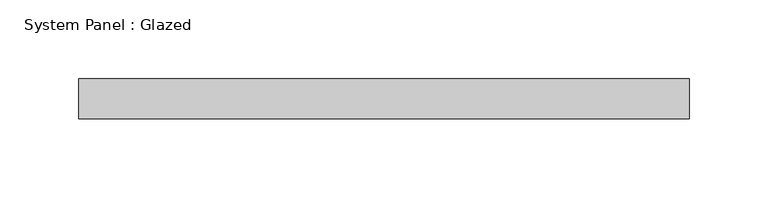
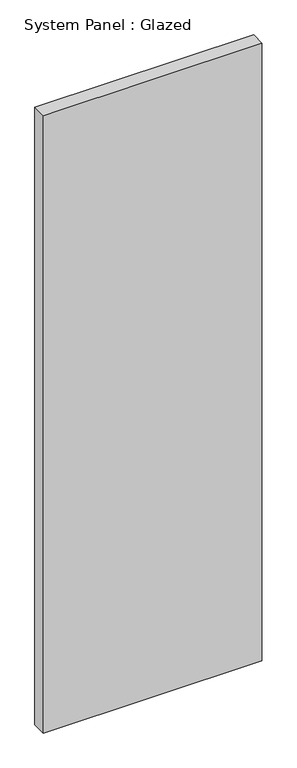
"""IFC4 building model written with IfcOpenShell, lengths in millimetres: plate geometry, System Panel : Glazed."""

from ifc_helpers import new_model, si_unit, origin, origin_with_axes, place, context, project, spatial, polyline, outline, extrude, source, transform, mapped, element, save


def system_panel_glazed_eddfd4ea(model_context):
    return source(origin(), model_context, "Body", "SweptSolid", [
        extrude(outline(polyline([(193.675, 19.05), (-193.675, 19.05), (-193.675, 44.45), (193.675, 44.45), (193.675, 19.05)])), origin_with_axes(), (0.0, 0.0, 1.0), 1155.7),
    ])


if __name__ == "__main__":
    model = new_model("IFC4")
    model_context = context("Model", 3, world=origin())
    ifc_project = project(units=[si_unit("LENGTHUNIT", "METRE", prefix="MILLI")], contexts=[model_context])
    site = spatial("IfcSite", under=ifc_project)
    building = spatial("IfcBuilding", under=site)
    placement = place(None, origin())
    system_panel_glazed_shape = system_panel_glazed_eddfd4ea(model_context)
    element("IfcPlate", 1, ObjectType="System Panel : Glazed", at=placement, inside=building, context=model_context, shape_type="MappedRepresentation", body=[
        mapped(system_panel_glazed_shape, transform((0.0, 0.0, 0.0), x_axis=(1.0, 0.0, 0.0), y_axis=(0.0, 1.0, 0.0), z_axis=(0.0, 0.0, 1.0))),
    ])
    save(model, "model.ifc")

# Revit data of these elements
# Type "System Panel : Glazed"
#   Construction Type Id = "GSP4R"
#   Analytic Construction = "1/8 in Pilkington single glazing"
#   Visual Light Transmittance = 0.9
#   Solar Heat Gain Coefficient = 0.86
#   Heat Transfer Coefficient (U) = 1.18115 BTU/(h·ft²·°F)
#   Define Thermal Properties by = 1
# Element 1 (IfcPlate, "System Panel : Glazed")
#   Materials on its faces: "Glass"
# Materials
#   "Glass": class "Glass", colour RGB 0 128 192, transparency 0.75, Description = "Soda Lime Glass", Cost = 0
